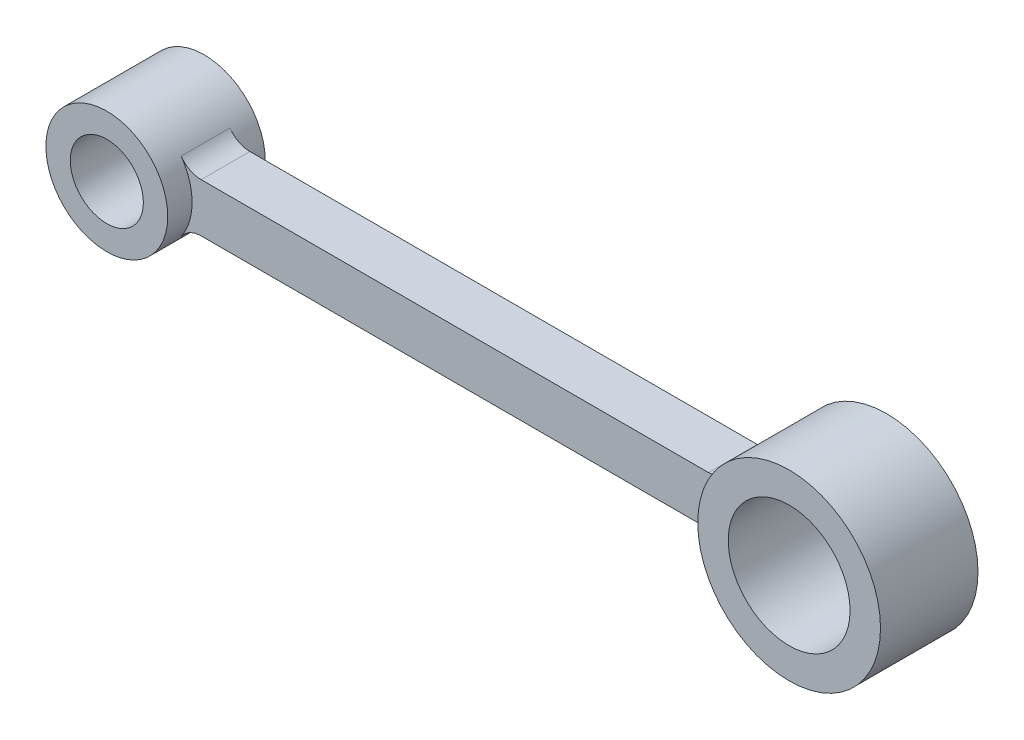
from build123d import *

# Parameters (mm, degrees)
ROD_PROFILE_SKETCH_R         = 5
ROD_PROFILE_SKETCH_R_2       = 3
ROD_BODY_EXTRUDE_8MM_DEPTH   = 4
ROD_PROFILE_SKETCH_R_3       = 7.5
ROD_BODY_EXTRUDE_8MM_2_DEPTH = 4
SHANK_BOSS_4MM_DEPTH         = 2
SHANK_FILLET_R2_R            = 2


with BuildPart() as part:
    # Rod Profile Sketch → Rod Body Extrude 8mm (new, symmetric)
    with BuildSketch(Plane.XY):
        with Locations((-29.25, 0)):
            Circle(ROD_PROFILE_SKETCH_R)
        with Locations((-29.25, 0)):
            Circle(ROD_PROFILE_SKETCH_R_2, mode=Mode.SUBTRACT)
    extrude(amount=ROD_BODY_EXTRUDE_8MM_DEPTH, both=True)



with BuildPart() as body_2:
    # Rod Profile Sketch → Rod Body Extrude 8mm 2 (new, symmetric)
    with BuildSketch(Plane.XY):
        with Locations((26.75, 0)):
            Circle(ROD_PROFILE_SKETCH_R_3)
        with Locations((26.75, 0)):
            Circle(ROD_PROFILE_SKETCH_R, mode=Mode.SUBTRACT)
    extrude(amount=ROD_BODY_EXTRUDE_8MM_2_DEPTH, both=True)


with BuildPart() as part_1:
    add(part.part)

    add(body_2.part)  # Shank Boss 4mm merges body 2
    # Shank Boss Sketch → Shank Boss 4mm (add, symmetric)
    with BuildSketch(Plane.XY):
        with BuildLine():
            Line((-24.667424305, 2), (19.521583853, 2))
            ThreePointArc((19.521583853, 2), (19.25, 0), (19.521583853, -2))
            Line((19.521583853, -2), (-24.667424305, -2))
            ThreePointArc((-24.667424305, -2), (-24.25, 0), (-24.667424305, 2))
        make_face()
    extrude(amount=SHANK_BOSS_4MM_DEPTH, both=True)

    # Shank Fillet R2
    shank_fillet_r2_edges = [part_1.edges().sort_by_distance(p)[0] for p in [
        (19.521583853, -2, 0),
        (19.521583853, 2, 0),
        (-24.667424305, 2, 0),
        (-24.667424305, -2, 0),
    ]]
    fillet(shank_fillet_r2_edges, radius=SHANK_FILLET_R2_R)


solid = part_1.part
